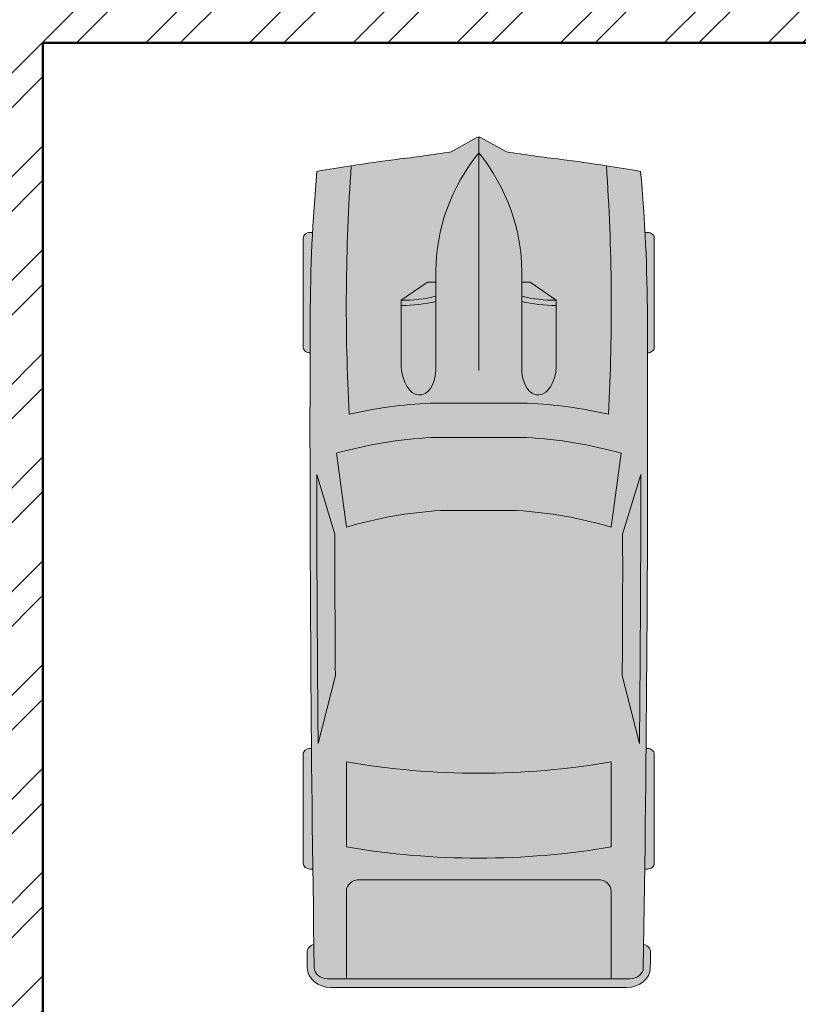
# Model space of a CAD drawing. Units: inches. Extents: x -31485 to -28799, y 18003 to 19130.
# Tile 2 of 15: x -30873 to -30771, y 18270 to 18398. Entities that reach past the tile are written whole.
import ezdxf

# ---------------------------------------------------------------- set-up
doc = ezdxf.new("R2010")
doc.units = ezdxf.units.IN
for name, color, linetype, lineweight in [('A-EQPM', 8, 'Continuous', 18), ('A-WALL', 7, 'Continuous', 50), ('A-WALL-PATT', 8, 'Continuous', 13)]:
    doc.layers.add(name, color=color, linetype=linetype, lineweight=lineweight)

# ---------------------------------------------------------------- blocks, each defined once
blk = doc.blocks.new('*U75')
for p, q in [((536.0433148737552, 950.1792138851854), (536.0433148737552, 935.5404748014407)), ((1182.463644577746, 987.7673041878503), (567.7039087844591, 987.7673041878503)), ((1214.124238488447, 949.7089586534819), (1214.124238488447, 950.1792138851854)), ((3440.463608272525, 941.6679440245914), (3440.463608272525, 950.1792138851854)), ((3472.124202183229, 987.7673041878503), (4086.88393797651, 987.767304187848)), ((4118.544531887212, 950.1792138851804), (4118.544531887212, 934.0601128753084)), ((2234.827175480885, 809.5287016048088), (1898.878785383111, 912.4126225124705)), ((3411.559256322833, 904.3494681924599), (3029.921878250559, 807.1504809911063)), ((4736.411271353851, -850.8646766016326), (4736.411271353883, 850.864676601626)), ((4785.334832293326, -832.0706314503777), (4785.334832293357, 832.0706314502926)), ((1778.76917512805, 801.0177247054045), (2194.716249451875, 745.5217224176465)), ((3515.941238262737, 745.5217224176508), (3994.062813016633, 745.5217224176508)), ((4736.411271353883, 745.5217224176529), (4242.012185201922, 745.5217224176529)), ((4178.690997380514, 670.345541812321), (4178.690997380509, -670.3455418123318)), ((819.5542361210883, 295.2827619512633), (917.6699264680983, 436.1082195367583)), ((917.6699264680983, 436.1082195367583), (1293.848362214069, 436.1082195367583)), ((815.9220749762081, 241.4481679439487), (815.9220749762081, 283.3039660446585)), ((756.2288711996046, 241.4481679439487), (1312.764151599097, 241.4481679439487)), ((1496.485716216861, -273.6820371142997), (1496.485716216861, 273.6820371142868)), ((1690.372337881975, -267.4332505757059), (1690.372337881975, 267.4332505756928)), ((4736.411271353883, -267.4332505757059), (4736.411271353883, 267.4332505756928)), ((2101.521373270556, 215.7994139342878), (2101.521373270556, -215.7994139342835)), ((82.96813941916749, 155.6585683733955), (2.596917328392246, 10.3141998552517)), ((-1.1252e-12, -6.4972e-12), (1312.764151599097, -6.4972e-12)), ((2.596917328392246, -10.31419985525964), (82.96813941916749, -155.6585683734063)), ((756.2288711996046, -241.4481679439617), (1312.764151599097, -241.4481679439617)), ((815.9220749762081, -241.4481679439617), (815.9220749762081, -283.3039660446715)), ((819.5542361210883, -295.2827619512763), (917.6699264680983, -436.1082195367712)), ((917.6699264680983, -436.1082195367712), (1293.848362214069, -436.1082195367712)), ((2194.716249451869, -745.5217224176688), (1778.769175128041, -801.0177247054262)), ((3994.062813016633, -745.5217224176616), (3515.941238262737, -745.5217224176638)), ((4242.012185201917, -745.5217224176638), (4736.411271353857, -745.5217224176594)), ((2234.827175480882, -809.5287016048153), (1898.878785383109, -912.4126225124726)), ((3411.559256322828, -904.349468192473), (3029.921878250557, -807.150480991115)), ((536.0433148737552, -950.1792138851984), (536.0433148737552, -935.5404748014537)), ((3440.463608272523, -941.6679440246044), (3440.463608272523, -950.1792138851984)), ((4118.544531887212, -950.1792138851933), (4118.544531887212, -934.0601128753214)), ((1182.463644577746, -987.7673041878633), (567.7039087844591, -987.7673041878633)), ((1214.124238488447, -949.7089586534948), (1214.124238488447, -950.1792138851984)), ((3472.124202183229, -987.7673041878633), (4086.883937976504, -987.767304187861))]:
    blk.add_line(p, q)
for centre, major_axis, ratio, start_param, end_param in [((1046.255263051279, -12467.92283887244), (3.2861e-12, 13417.14359589015), 0.8423038695439741, 0.0028100083536837, 0.0755983031096952), ((567.7039087844591, 950.1792138851861), (5.296e-13, -37.5880903026662), 0.842303869543976, 3.141592653589776, 4.712388980384677), ((1637.842620806017, -268112.68896731), (4.8454159e-09, 269062.8681811952), 0.842303869543847, -0.0133969486112073, 0.0027970409639888), ((1182.463644577746, 950.1792138851861), (5.601e-13, 37.58809030266621), 0.8423038695439758, -1.570796326794884, 1.73e-14), ((3472.124202183229, 950.1792138851861), (5.988e-12, -37.5880903026662), 0.8423038695439762, 3.141592653589603, 4.712388980384554), ((4086.88393797651, 950.179213885181), (1.4197e-12, 37.5880903026662), 0.842303869543976, -1.570796326794865, 4.44e-14), ((4587.952203166941, 910.2894362332722), (1.8792e-12, 56.38213545399769), 0.8423038695439691, -0.0130174256259048, 1.249894140392862), ((1637.84262086767, -268131.4830124673), (3.42859201765e-05, 269120.9512111412), 0.8423038681351471, -0.0133969484821159, -0.0130174254969711), ((4673.090083532448, 832.070631450172), (2.1733e-12, -133.2592106239272), 0.8423038695439737, 1.570796326795794, 3.128195704978164), ((6757.162543998887, -699.1204428451242), (4.9938223e-09, 7958.017136535005), 0.8423038695435286, 1.367075990158062, 1.391760499156098), ((1637.842620802809, -268112.6889680619), (4.87113144e-08, -269025.2800916445), 0.8423038695482963, 3.133765086725325, 3.140440689641252), ((4673.090083532475, 850.8646766015395), (7.5e-15, -75.17618060533067), 0.8423038695439952, 1.570796326796048, 3.128195704978389), ((3436.395912346701, 136.8410185571553), (5.76965e-11, 2077.023647078763), 0.8423038695439563, 1.245306111696802, 1.507880129813836), ((2433.035484508693, -93125.37499596032), (4.952654e-09, -93935.19844392464), 0.8423038695446962, 3.134048706297306, 3.14409775411291), ((951.8333444315502, -15086.63944974413), (1.5767e-12, -15832.53653317094), 0.8423038695439826, 3.09604606856106, 3.200911180495224), ((3413.769624379244, 136.8410185571329), (1.08602e-11, -2280.347340451234), 0.84230386954398, 4.44948196380473, 4.652344057257214), ((3799.722190048092, 71.1058404433382), (2.17448e-11, -2021.323467232052), 0.842303869543983, 4.372215489277867, 4.640744122441986), ((433.884764992104, -3.6096e-12), (1.7438e-12, 3734.255266801694), 0.8423038695439766, 4.511394369635731, 4.913383591133647), ((912.0063397460013, -3.6096e-12), (1.7438e-12, 3734.255266801694), 0.8423038695439766, 4.511394369635731, 4.913383591133647), ((4242.012185201922, 670.3455418123216), (3.5405e-12, 75.17618060533239), 0.842303869543976, 5.55e-14, 1.57079632679492), ((6583.045501169266, -699.1204428451198), (3.826807e-09, -7754.693443154298), 0.8423038695443791, 4.528606069860317, 4.561837674556238), ((-5194.164488957196, 1330.879982200552), (1.0466145e-09, -6374.389491984369), 0.8423038695441164, 1.385369446298923, 1.434372047871027), ((331.12799165183, 432.0470009052715), (3.125e-11, 696.3661584994836), 0.8423038695439277, 4.435146050259648, 4.718221029521873), ((360.7019022476185, 432.0470009052715), (3.125e-11, 696.3661584994836), 0.8423038695439277, 4.435146050259648, 4.718221029521873), ((1290.073045555822, 338.7781937403542), (161.0379696969085, -9.057857958340485), 0.6038335755719145, -1.39555193967809, 1.581314658479915), ((831.7523719315589, 283.3039660446593), (3.3347e-12, 18.79404515133458), 0.8423038695439091, 0.8797135699495516, 1.570796326795045), ((756.2288711996046, -1185.240851913765), (1.2998e-12, 1426.689019857713), 0.842303869543976, 7e-16, 0.5903187773915901), ((15.83029695535095, -3.6096e-12), (1.9e-15, -18.79404515133476), 0.842303869543842, 4.131459131953847, 5.293318828815531), ((756.2288711996046, 1185.240851913753), (1.01699e-11, 1426.689019857713), 0.8423038695439736, 2.55127387619821, 3.141592653589801), ((-5194.164488957196, -1330.879982200562), (1.0234792e-09, 6374.389491984348), 0.8423038695441192, -1.43437204787103, -1.385369446298926), ((3799.722190048497, -71.10584044329416), (1.038796e-10, -2021.323467232635), 0.8423038695439419, -1.499151468852248, -1.230622835688196), ((331.12799165183, -432.0470009052816), (3.1922e-11, -696.3661584994801), 0.842303869543932, 1.564964277657711, 1.848039256919935), ((360.7019022476185, -432.0470009052816), (3.1922e-11, -696.3661584994801), 0.842303869543932, 1.564964277657711, 1.848039256919935), ((3413.769624379237, -136.841018557156), (1.090899e-10, -2280.347340451348), 0.8423038695439354, -1.510751403667474, -1.307889310215002), ((3436.395912346742, -136.8410185572101), (8.13766e-11, -2077.023647078826), 0.8423038695439492, -1.50788012981387, -1.245306111696839), ((831.7523719315589, -283.3039660446737), (3.3028e-12, -18.79404515133458), 0.8423038695439093, 4.712388980384541, 5.403471737230034), ((6583.045501169163, 699.1204428449458), (2.756795e-10, 7754.693443157768), 0.8423038695439974, 1.721347632622872, 1.754579237318777), ((6757.162543998887, 699.1204428451076), (2.2231118e-09, 7958.017136528592), 0.8423038695441819, 1.749832154434603, 1.774516663432659), ((951.8333444315729, 15086.63944974408), (2.97009e-11, -15832.5365331709), 0.8423038695439528, -0.0593185269054384, 0.0455465850287298), ((4242.012185201917, -670.3455418123318), (2.579e-13, -75.17618060533128), 0.8423038695439885, 4.712388980384686, 6.283185307179581), ((2433.03548450906, 93125.37499596029), (4.1600574e-09, -93935.19844392457), 0.8423038695447548, -0.0025051005232382, 0.007543947292366), ((4673.090083532448, -850.8646766015358), (2.354e-13, 75.17618060532999), 0.8423038695439732, 3.154989602201626, 4.71238898038339), ((4673.090083532349, -832.0706314501077), (6.1679e-12, -133.2592106240062), 0.8423038695439807, 0.0133969486110846, 1.570796326792831), ((1046.255263051284, 12467.92283887242), (3.49903e-10, -13417.14359589015), 0.8423038695440652, -0.0755983031097181, -0.0028100083537155), ((1637.842620801787, 268112.6889680619), (1.55395844e-08, 269062.868181947), 0.8423038695458147, 3.138795612625926, 3.154989602201039), ((1637.842620803916, 268112.6889680615), (4.0766478e-08, -269025.280091644), 0.8423038695397146, 0.0011519639481523, 0.0078275668641468), ((4587.952203166856, -910.2894362333229), (5.777e-12, -56.38213545402103), 0.8423038695439803, -1.249894138785958, 0.0130174256254374), ((567.7039087844591, -950.1792138851977), (5.601e-13, 37.58809030266621), 0.8423038695439758, 1.570796326794908, 3.14159265358981), ((1182.463644577746, -950.1792138851977), (5.296e-13, -37.5880903026662), 0.842303869543976, -1.69e-14, 1.570796326794884), ((3472.124202183229, -950.1792138851955), (3.96e-13, -37.58809030266733), 0.8423038695440105, -1.570796326794875, -1.27e-14), ((4086.883937976504, -950.1792138851933), (5.0003e-12, 37.58809030266732), 0.8423038695440109, 3.141592653589951, 4.712388980384771), ((1637.842620726191, 268131.4830135791), (2.37878358395e-05, 269120.9512123862), 0.8423038705260315, 3.154610079306566, 3.154989602290631)]:
    blk.add_ellipse(centre, major_axis=major_axis, ratio=ratio, start_param=start_param, end_param=end_param)
at = {"extrusion": (0, 0, -1)}
blk.add_ellipse((1290.073045555822, -338.7781937403665), major_axis=(161.0379696969085, 9.057857958340424), ratio=0.6038335755719145, start_param=-1.39555193967809, end_param=1.581314658479915, dxfattribs=at)

msp = doc.modelspace()

# ---------------------------------------------------------------- hatches: boundary and pattern name
at = {"layer": 'A-EQPM'}
h = msp.add_hatch(color=256, dxfattribs=at)
h.dxf.hatch_style = 1
edge = h.paths.add_edge_path()
edge.add_ellipse((-30809.74980735968, 18303.27344922968), major_axis=(-47.91849192778267, 1.361529e-10), ratio=0.8423038695419347, start_angle=248.1650462034528, end_angle=265.722579037107)
edge.add_line((-30806.7369467095, 18343.55552145171), (-30819.07671768603, 18343.55552145171))
edge.add_ellipse((-30816.06385703584, 18303.27344922968), major_axis=(47.91849192778146, 1.460375e-10), ratio=0.8423038695419556, start_angle=94.277420962876, end_angle=111.8349537965306)
edge.add_line((-30831.3869113385, 18341.51614017747), (-30830.10657698055, 18331.91992948851))
edge.add_ellipse((-30814.54729721899, 18294.89123974947), major_axis=(46.63344704056234, 1.445442e-10), ratio=0.842303869541784, start_angle=94.8700695969602, end_angle=112.7919148774121, ccw=False)
edge.add_line((-30817.8854863836, 18334.07000511634), (-30807.92817801193, 18334.07000511634))
edge.add_ellipse((-30811.26636717653, 18294.89123974948), major_axis=(-46.63344704055716, 1.546607e-10), ratio=0.8423038695417213, start_angle=247.20808512260112, end_angle=265.1299304030565, ccw=False)
edge.add_line((-30795.70708741497, 18331.91992948851), (-30794.42675305702, 18341.51614017747))
edge = h.paths.add_edge_path()
edge.add_ellipse((-30840.2512267956, 18365.10691121584), major_axis=(-32.91478475822442, 2.78257e-11), ratio=0.8423038695443898, start_angle=180.0000000000484, end_angle=209.4385695980319)
edge.add_ellipse((-30785.56243759992, 18365.10691121584), major_axis=(32.91478475822442, 2.78184e-11), ratio=0.8423038695443903, start_angle=150.561430401968, end_angle=179.9999999999515)
edge.add_line((-30818.47722235815, 18365.10691121584), (-30818.47722235815, 18352.26722526484))
edge.add_ellipse((-30820.72269898621, 18352.79072608453), major_axis=(-0.2089715704820894, 3.715266632531377), ratio=0.6038335755718302, start_angle=89.0020142750023, end_angle=253.6574080457279, ccw=False)
edge.add_line((-30822.96817561427, 18352.70362670025), (-30822.96817561427, 18361.38234509712))
edge.add_line((-30822.96817561427, 18361.38234509712), (-30819.64068913299, 18363.70066622193))
edge.add_ellipse((-30819.44286698441, 18363.36452746144), major_axis=(0.4335927047225755, 4.12191e-11), ratio=0.8423038695061222, start_angle=89.99999999455332, end_angle=134.4802108771379, ccw=False)
edge.add_line((-30819.44286698441, 18363.72974427442), (-30818.47722235815, 18363.72974427442))
edge.add_line((-30818.47722235815, 18363.72974427442), (-30818.47722235815, 18365.10691121584))
edge.add_ellipse((-30785.56243759992, 18365.10691121584), major_axis=(32.91478475822442, 2.78184e-11), ratio=0.8423038695443903, start_angle=150.5614304019681, end_angle=179.9999999999516, ccw=False)
edge.add_line((-30812.90683219776, 18380.53894657792), (-30812.90683219776, 18382.55367794428))
edge.add_ellipse((-30812.90683219776, 18382.18846113131), major_axis=(-0.4335927046986816, 0), ratio=0.842303869552539, start_angle=270, end_angle=307.9331304600232)
edge.add_line((-30813.14478851723, 18382.49376511555), (-30816.49799201077, 18380.63954079683))
edge.add_ellipse((-30843.61123066403, 18502.38694488138), major_axis=(-147.0619421372835, 4.9907306e-09), ratio=0.8423038695736066, start_angle=99.2565660091451, end_angle=102.55493264608151, ccw=False)
edge.add_ellipse((-30796.77759970489, 18230.67788531626), major_axis=(178.9065886092977, 1.2789651e-09), ratio=0.8423038695391513, start_angle=100.209538996733, end_angle=102.4446272930335)
edge.add_ellipse((-30464.84675512309, 18360.59416944481), major_axis=(365.2684817172171, 7.18011e-11), ratio=0.8423038695434502, start_angle=177.1362853921513, end_angle=182.1985405659441)
edge.add_ellipse((-30816.06385703584, 18303.79545464779), major_axis=(52.60932189168197, 7.16232e-11), ratio=0.8423038695431074, start_angle=94.08241069107589, end_angle=107.71995322267611, ccw=False)
edge.add_line((-30819.22088187392, 18348.02863109984), (-30806.59278252161, 18348.02863109984))
edge.add_ellipse((-30809.74980735968, 18303.79545464779), major_axis=(-52.6093218916263, 2.96862e-11), ratio=0.842303869543985, start_angle=252.2800467772827, end_angle=265.9175893088832, ccw=False)
edge.add_ellipse((-31160.96690927244, 18360.59416944481), major_axis=(365.2684817172168, 5.54988e-11), ratio=0.8423038695419378, start_angle=-2.198540565964143, end_angle=2.863714607828726)
edge.add_ellipse((-30829.03606469064, 18230.67788531626), major_axis=(-178.9065886093012, 1.2581094e-09), ratio=0.8423038695391548, start_angle=257.5553727069574, end_angle=259.7904610032577)
edge.add_ellipse((-30782.2024337315, 18502.38694488138), major_axis=(147.0619421407358, 1.9919546e-09), ratio=0.8423038695542743, start_angle=257.4450673550873, end_angle=260.74343399202326, ccw=False)
edge.add_line((-30809.31567238475, 18380.63954079683), (-30812.6688758783, 18382.49376511555))
edge.add_ellipse((-30812.90683219776, 18382.18846113131), major_axis=(-0.4335927046986816, 0), ratio=0.842303869552539, start_angle=232.0668695399768, end_angle=270)
edge.add_line((-30812.90683219776, 18382.55367794428), (-30812.90683219776, 18380.53894657792))
edge.add_ellipse((-30840.2512267956, 18365.10691121584), major_axis=(-32.91478475822442, 2.78257e-11), ratio=0.8423038695443898, start_angle=180.0000000000485, end_angle=209.438569598032, ccw=False)
edge.add_line((-30807.33644203738, 18365.10691121584), (-30807.33644203738, 18363.72974427442))
edge.add_line((-30807.33644203738, 18363.72974427442), (-30806.21471099341, 18363.72974427442))
edge.add_line((-30806.21471099341, 18363.72974427442), (-30802.84548878126, 18361.38234509712))
edge.add_line((-30802.84548878126, 18361.38234509712), (-30802.84548878126, 18352.70362670025))
edge.add_ellipse((-30805.09096540932, 18352.79072608453), major_axis=(0.2089715704820894, 3.715266632531377), ratio=0.6038335755718302, start_angle=106.3425919542722, end_angle=270.9979857249977, ccw=False)
edge.add_line((-30807.33644203738, 18352.26722526484), (-30807.33644203738, 18365.10691121584))
edge = h.paths.add_edge_path()
edge.add_ellipse((-28664.43464880163, 18326.42172615445), major_axis=(-2167.155417170912, 9.004676e-10), ratio=0.8423038695746358, start_angle=-0.12089736900918524, end_angle=0.3640763489138976, ccw=False)
edge.add_line((-30831.58326595316, 18330.99454036844), (-30833.95687510317, 18338.74512146637))
edge.add_ellipse((-24627.34619108991, 18344.76742138713), major_axis=(6206.614802166701, 5.2511138e-09), ratio=0.842303869515611, start_angle=180.0555943134505, end_angle=180.377764193861)
edge.add_line((-30833.77085209099, 18303.84644949518), (-30831.52839862151, 18312.65110978209))
edge = h.paths.add_edge_path()
edge.add_ellipse((-36998.46747330562, 18344.76742138716), major_axis=(-6206.61480216671, 6.192387e-09), ratio=0.8423038695127218, start_angle=179.6222358061472, end_angle=179.9444056865578)
edge.add_line((-30791.85678929235, 18338.74512146637), (-30794.23039844237, 18330.99454036844))
edge.add_ellipse((-32961.37901559391, 18326.42172615446), major_axis=(-2167.155417170919, 1.3253717e-09), ratio=0.8423038695188795, start_angle=179.6359236511448, end_angle=180.1208973690678, ccw=False)
edge.add_line((-30794.28526577401, 18312.65110978209), (-30792.04281230453, 18303.84644949516))
edge = h.paths.add_edge_path()
edge.add_ellipse((-30812.90683219776, 18372.54363129024), major_axis=(-86.15206721880882, 2.44e-14), ratio=0.8423038695434939, start_angle=76.40186530976911, end_angle=103.598134690231, ccw=False)
edge.add_line((-30830.10657698055, 18301.43827895458), (-30830.10657698055, 18290.40765595108))
edge.add_ellipse((-30812.90683219776, 18361.51300828673), major_axis=(-86.15206721880666, 5.3e-15), ratio=0.8423038695434728, start_angle=76.40186530976838, end_angle=103.5981346902316)
edge.add_line((-30795.70708741497, 18290.40765595108), (-30795.70708741497, 18301.43827895458))
edge = h.paths.add_edge_path()
edge.add_ellipse((-30797.44145823379, 18284.68727813726), major_axis=(-1.734370818820025, 1.15572e-11), ratio=0.8423038695444475, start_angle=180.0000000003817, end_angle=270.0000000003818)
edge.add_line((-30797.44145823379, 18286.14814538917), (-30828.37220616173, 18286.14814538917))
edge.add_ellipse((-30828.37220616173, 18284.68727813726), major_axis=(1.734370818820025, 1.15576e-11), ratio=0.8423038695444475, start_angle=89.99999999961817, end_angle=179.9999999996181)
edge.add_line((-30830.10657698055, 18284.68727813726), (-30830.10657698055, 18273.28112074847))
edge.add_line((-30830.10657698055, 18273.28112074847), (-30795.70708741497, 18273.28112074847))
edge.add_line((-30795.70708741497, 18273.28112074847), (-30795.70708741497, 18284.68727813726))
h = msp.add_hatch(color=256, dxfattribs=at)
h.dxf.hatch_style = 1
edge = h.paths.add_edge_path()
edge.add_ellipse((-36998.46747328827, 18344.76742138709), major_axis=(6207.481987558777, 4.152598e-10), ratio=0.8423038695472291, start_angle=-0.3838667787963557, end_angle=0.0902290885904627)
edge.add_ellipse((-36998.46747328827, 18344.76742138709), major_axis=(6207.481987558777, 4.152598e-10), ratio=0.8423038695472291, start_angle=0.0902290885904627, end_angle=0.1349865768543979)
edge.add_ellipse((-31100.55115475978, 18358.41578502847), major_axis=(309.5435567121417, 3.12922e-11), ratio=0.8423038695440732, start_angle=0.1806905311799308, end_angle=2.179950313639523)
edge.add_ellipse((-31100.55115475978, 18358.41578502847), major_axis=(309.5435567121417, 3.12922e-11), ratio=0.8423038695440732, start_angle=2.179950313639523, end_angle=3.650427585692763)
edge.add_ellipse((-30829.03606469064, 18226.66087466593), major_axis=(183.5974185536168, 2.07254122e-08), ratio=0.8423038696260594, start_angle=76.2194710040335, end_angle=77.87403444124779)
edge.add_ellipse((-31160.96690927244, 18360.59416944481), major_axis=(365.2684817172168, 5.54988e-11), ratio=0.8423038695419378, start_angle=-2.1985405659640946, end_angle=2.8637146078286833, ccw=False)
edge.add_ellipse((-30809.74980735968, 18303.79545464779), major_axis=(-52.6093218916263, 2.96862e-11), ratio=0.842303869543985, start_angle=252.2800467772827, end_angle=265.9175893088831)
edge.add_line((-30806.59278252161, 18348.02863109984), (-30819.22088187392, 18348.02863109984))
edge.add_ellipse((-30816.06385703584, 18303.79545464779), major_axis=(52.60932189168197, 7.16232e-11), ratio=0.8423038695431074, start_angle=94.08241069107586, end_angle=107.719953222676)
edge.add_ellipse((-30464.84675512309, 18360.59416944481), major_axis=(365.2684817172171, 7.18011e-11), ratio=0.8423038695434502, start_angle=177.1362853921513, end_angle=182.1985405659441, ccw=False)
edge.add_ellipse((-30796.77759970488, 18226.66087466593), major_axis=(-183.5974185535601, 2.07797544e-08), ratio=0.8423038696263095, start_angle=-77.87403444123211, end_angle=-76.21947100401783)
edge.add_ellipse((-30525.26250963575, 18358.41578502847), major_axis=(-309.5435567121417, 3.20483e-11), ratio=0.8423038695440663, start_angle=-3.650427585692615, end_angle=-2.179950313639383)
edge.add_ellipse((-30525.26250963575, 18358.41578502847), major_axis=(-309.5435567121417, 3.20483e-11), ratio=0.8423038695440663, start_angle=-2.179950313639383, end_angle=-0.1356123904320413)
edge.add_ellipse((-24627.3461910899, 18344.76742138718), major_axis=(6207.481987576122, 7.89454e-11), ratio=0.842303869542251, start_angle=179.8650134231422, end_angle=179.9097709114061)
edge.add_ellipse((-24627.3461910899, 18344.76742138718), major_axis=(6207.481987576122, 7.89454e-11), ratio=0.842303869542251, start_angle=179.9097709114061, end_angle=180.3838667787915)
edge.add_ellipse((-24627.3461910899, 18344.76742138718), major_axis=(6207.481987576122, 7.89454e-11), ratio=0.842303869542251, start_angle=180.3838667787915, end_angle=180.5282714718166)
edge.add_ellipse((-24627.3461910899, 18344.76742138718), major_axis=(6207.481987576122, 7.89454e-11), ratio=0.842303869542251, start_angle=180.5282714718166, end_angle=180.6465540970602)
edge.add_ellipse((-30832.53691787089, 18274.74198800039), major_axis=(1.734370818820398, 6.2835e-12), ratio=0.8423038695442665, start_angle=180.6465540968934, end_angle=269.9999999996497)
edge.add_line((-30832.53691787089, 18273.28112074847), (-30830.10657698055, 18273.28112074847))
edge.add_line((-30830.10657698055, 18273.28112074847), (-30830.10657698055, 18285.22199266301))
edge.add_ellipse((-30828.37220616173, 18284.68727813726), major_axis=(1.734370818820025, 1.15576e-11), ratio=0.8423038695444475, start_angle=89.99999999961818, end_angle=179.9999999996182, ccw=False)
edge.add_line((-30828.37220616173, 18286.14814538917), (-30796.80663445453, 18286.14814538917))
edge.add_ellipse((-30797.44145823379, 18284.68727813726), major_axis=(-1.734370818820025, 1.15572e-11), ratio=0.8423038695444475, start_angle=180.0000000003818, end_angle=270.00000000038176, ccw=False)
edge.add_line((-30795.70708741497, 18284.68727813726), (-30795.70708741497, 18273.28112074847))
edge.add_line((-30795.70708741497, 18273.28112074847), (-30793.27674652463, 18273.28112074847))
edge.add_ellipse((-30793.27674652464, 18274.74198800038), major_axis=(-1.734370818820364, 1.2413e-12), ratio=0.8423038695421853, start_angle=90.00000000018369, end_angle=179.3534459030602)
edge.add_ellipse((-36998.46747328827, 18344.76742138709), major_axis=(6207.481987558777, 4.152598e-10), ratio=0.8423038695472291, start_angle=-0.6465540970657812, end_angle=-0.618643196323059)
edge.add_ellipse((-36998.46747328827, 18344.76742138709), major_axis=(6207.481987558777, 4.152598e-10), ratio=0.8423038695472291, start_angle=-0.618643196323059, end_angle=-0.528271471821792)
edge.add_ellipse((-36998.46747328827, 18344.76742138709), major_axis=(6207.481987558777, 4.152598e-10), ratio=0.8423038695472291, start_angle=-0.528271471821792, end_angle=-0.3838667787963557)
edge = h.paths.add_edge_path(flags=16)
edge.add_ellipse((-30814.54729721899, 18294.89123974947), major_axis=(46.63344704056234, 1.445442e-10), ratio=0.842303869541784, start_angle=94.8700695969603, end_angle=112.7919148774121)
edge.add_line((-30830.10657698055, 18331.91992948851), (-30831.3869113385, 18341.51614017747))
edge.add_ellipse((-30816.06385703584, 18303.27344922968), major_axis=(47.91849192778146, 1.460375e-10), ratio=0.8423038695419556, start_angle=94.27742096287608, end_angle=111.8349537965307, ccw=False)
edge.add_line((-30819.07671768603, 18343.55552145171), (-30806.7369467095, 18343.55552145171))
edge.add_ellipse((-30809.74980735968, 18303.27344922968), major_axis=(-47.91849192778267, 1.361529e-10), ratio=0.8423038695419347, start_angle=248.1650462034528, end_angle=265.72257903710704, ccw=False)
edge.add_line((-30794.42675305702, 18341.51614017747), (-30795.70708741497, 18331.91992948851))
edge.add_ellipse((-30811.26636717653, 18294.89123974948), major_axis=(-46.63344704055716, 1.546607e-10), ratio=0.8423038695417213, start_angle=247.208085122601, end_angle=265.1299304030565)
edge.add_line((-30807.92817801193, 18334.07000511634), (-30817.8854863836, 18334.07000511634))
edge = h.paths.add_edge_path(flags=16)
edge.add_line((-30794.23039844237, 18330.99454036844), (-30791.85678929235, 18338.74512146637))
edge.add_ellipse((-36998.46747330562, 18344.76742138716), major_axis=(-6206.61480216671, 6.192387e-09), ratio=0.8423038695127218, start_angle=179.6222358061473, end_angle=179.9444056865578, ccw=False)
edge.add_line((-30792.04281230453, 18303.84644949516), (-30794.28526577401, 18312.65110978209))
edge.add_ellipse((-32961.37901559391, 18326.42172615446), major_axis=(-2167.155417170919, 1.3253717e-09), ratio=0.8423038695188795, start_angle=179.6359236511447, end_angle=180.1208973690677)
edge = h.paths.add_edge_path(flags=16)
edge.add_ellipse((-28664.43464880163, 18326.42172615445), major_axis=(-2167.155417170912, 9.004676e-10), ratio=0.8423038695746358, start_angle=-0.1208973690091865, end_angle=0.364076348913875)
edge.add_line((-30831.52839862151, 18312.65110978209), (-30833.77085209099, 18303.84644949518))
edge.add_ellipse((-24627.34619108991, 18344.76742138713), major_axis=(6206.614802166701, 5.2511138e-09), ratio=0.842303869515611, start_angle=180.0555943134506, end_angle=180.3777641938611, ccw=False)
edge.add_line((-30833.95687510317, 18338.74512146637), (-30831.58326595316, 18330.99454036844))
edge = h.paths.add_edge_path(flags=16)
edge.add_ellipse((-30812.90683219776, 18372.54363129024), major_axis=(-86.15206721880882, 2.44e-14), ratio=0.8423038695434939, start_angle=76.40186530976904, end_angle=103.5981346902309)
edge.add_line((-30795.70708741497, 18301.43827895458), (-30795.70708741497, 18290.40765595108))
edge.add_ellipse((-30812.90683219776, 18361.51300828673), major_axis=(-86.15206721880666, 5.3e-15), ratio=0.8423038695434728, start_angle=76.40186530976843, end_angle=103.59813469023157, ccw=False)
edge.add_line((-30830.10657698055, 18290.40765595108), (-30830.10657698055, 18301.43827895458))
h = msp.add_hatch(color=256, dxfattribs=at)
h.dxf.hatch_style = 1
edge = h.paths.add_edge_path()
edge.add_ellipse((-30802.9391841383, 18374.9143070506), major_axis=(-16.06568908915088, 3.60949e-11), ratio=0.8423038695435023, start_angle=71.33250450753093, end_angle=90.39670986011208, ccw=False)
edge.add_line((-30807.33644203738, 18361.89885908758), (-30807.33644203738, 18361.21656680932))
edge.add_ellipse((-30802.9391841383, 18374.23201477234), major_axis=(16.06568908904641, 9.1463e-11), ratio=0.8423038695487669, start_angle=251.332504507076, end_angle=270.3967098596572)
edge.add_line((-30802.84548878126, 18360.70005281887), (-30802.84548878126, 18361.38234509712))
edge = h.paths.add_edge_path()
edge.add_ellipse((-30822.87448025722, 18374.9143070506), major_axis=(16.06568908915091, 3.60949e-11), ratio=0.8423038695435009, start_angle=269.6032901398879, end_angle=288.667495492469, ccw=False)
edge.add_line((-30822.96817561427, 18361.38234509712), (-30822.96817561427, 18360.70005281887))
edge.add_ellipse((-30822.87448025722, 18374.23201477234), major_axis=(-16.06568908904639, 9.1463e-11), ratio=0.8423038695487673, start_angle=89.60329014034272, end_angle=108.667495492924)
edge.add_line((-30818.47722235815, 18361.21656680932), (-30818.47722235815, 18361.89885908758))
edge = h.paths.add_edge_path()
edge.add_ellipse((-30790.9854857295, 18369.45632336739), major_axis=(0.8671854094100124, 1.6795e-12), ratio=0.8423038695444477, start_angle=-1.109639e-10, end_angle=89.99999999988906)
edge.add_line((-30790.9854857295, 18370.18675699335), (-30791.3232124095, 18370.18675699335))
edge.add_ellipse((-31100.55115475978, 18358.41578502847), major_axis=(309.5435567121417, 3.12922e-11), ratio=0.8423038695440732, start_angle=0.18069053117989142, end_angle=2.1799503136394947, ccw=False)
edge.add_ellipse((-31100.55115475978, 18358.41578502847), major_axis=(309.5435567121417, 3.12922e-11), ratio=0.8423038695440732, start_angle=0.1356123904321862, end_angle=0.18069053117989142, ccw=False)
edge.add_ellipse((-36998.46747328827, 18344.76742138709), major_axis=(6207.481987558777, 4.152598e-10), ratio=0.8423038695472291, start_angle=0.09022908859049039, end_angle=0.13498657685437365, ccw=False)
edge.add_line((-30790.99633487007, 18354.54292197479), (-30790.9854857295, 18354.54292197479))
edge.add_ellipse((-30790.9854857295, 18355.27335560075), major_axis=(-0.8671854094100128, 1.6795e-12), ratio=0.8423038695444475, start_angle=90.00000000011094, end_angle=180.0000000001109)
edge.add_line((-30790.11830032009, 18355.27335560075), (-30790.11830032009, 18369.45632336739))
edge = h.paths.add_edge_path()
edge.add_ellipse((-30525.26250963575, 18358.41578502847), major_axis=(-309.5435567121417, 3.20483e-11), ratio=0.8423038695440663, start_angle=-2.179950313639381, end_angle=-0.13561239043201567, ccw=False)
edge.add_line((-30834.49045198602, 18370.18675699335), (-30834.82817866603, 18370.18675699335))
edge.add_ellipse((-30834.82817866603, 18369.45632336739), major_axis=(-0.8671854094100128, 1.6795e-12), ratio=0.8423038695444475, start_angle=-89.99999999988903, end_angle=1.109639e-10)
edge.add_line((-30835.69536407544, 18369.45632336739), (-30835.69536407544, 18355.27335560075))
edge.add_ellipse((-30834.82817866603, 18355.27335560075), major_axis=(0.8671854094100124, 1.6795e-12), ratio=0.8423038695444477, start_angle=179.999999999889, end_angle=269.999999999889)
edge.add_line((-30834.82817866603, 18354.54292197479), (-30834.81732952545, 18354.54292197479))
edge.add_ellipse((-24627.3461910899, 18344.76742138718), major_axis=(6207.481987576122, 7.89454e-11), ratio=0.842303869542251, start_angle=179.8650134231423, end_angle=179.9097709114062, ccw=False)
edge = h.paths.add_edge_path()
edge.add_ellipse((-30793.71033922934, 18274.74198800039), major_axis=(3.074389845080431, 4.5193e-12), ratio=0.8423038695441155, start_angle=269.9999999999962, end_angle=359.3534459027799)
edge.add_ellipse((-36998.90106599311, 18344.76742138567), major_axis=(6208.822006597157, 5.2733581016e-06), ratio=0.8423038788855699, start_angle=-0.6465541457119849, end_angle=-0.6282372648788389)
edge.add_ellipse((-30791.90577279079, 18276.70618269733), major_axis=(-1.30077811411332, 2.65586e-11), ratio=0.8423038695457158, start_angle=179.3717627849924, end_angle=248.4647566023133)
edge.add_ellipse((-36998.46747328827, 18344.76742138709), major_axis=(6207.481987558777, 4.152598e-10), ratio=0.8423038695472291, start_angle=-0.6465540970658026, end_angle=-0.6186431963230916, ccw=False)
edge.add_ellipse((-30793.27674652464, 18274.74198800038), major_axis=(-1.734370818820364, 1.2413e-12), ratio=0.8423038695421853, start_angle=90.00000000018372, end_angle=179.3534459030602, ccw=False)
edge.add_line((-30793.27674652463, 18273.28112074847), (-30832.53691787089, 18273.28112074847))
edge.add_ellipse((-30832.53691787089, 18274.74198800039), major_axis=(1.734370818820398, 6.2835e-12), ratio=0.8423038695442665, start_angle=180.6465540968934, end_angle=269.99999999964973, ccw=False)
edge.add_ellipse((-24627.3461910899, 18344.76742138718), major_axis=(6207.481987576122, 7.89454e-11), ratio=0.842303869542251, start_angle=180.5282714718167, end_angle=180.6465540970602, ccw=False)
edge.add_ellipse((-30833.90789160473, 18276.70618269733), major_axis=(1.300778114113422, 3.7711e-12), ratio=0.8423038695465029, start_angle=111.5352435038071, end_angle=180.6282372160113)
edge.add_ellipse((-24626.91259837676, 18344.76742138893), major_axis=(-6208.822006624284, 5.909233014e-06), ratio=0.842303880027109, start_angle=0.6282372707742053, end_angle=0.6465541516072572)
edge.add_ellipse((-30832.10332516618, 18274.74198800039), major_axis=(-3.074389845084005, 2.9376e-12), ratio=0.8423038695431365, start_angle=0.6465540971220629, end_angle=89.99999999989375)
edge.add_line((-30832.10332516619, 18272.15241753739), (-30793.71033922934, 18272.15241753739))
edge = h.paths.add_edge_path()
edge.add_ellipse((-24627.3461910899, 18344.76742138718), major_axis=(6207.481987576122, 7.89454e-11), ratio=0.842303869542251, start_angle=180.3838667787916, end_angle=180.5282714718167, ccw=False)
edge.add_line((-30834.63181729253, 18303.1796044366), (-30834.82817866603, 18303.1796044366))
edge.add_ellipse((-30834.82817866603, 18302.44917081064), major_axis=(-0.8671854094100128, 1.6795e-12), ratio=0.8423038695444475, start_angle=-89.99999999988903, end_angle=1.109639e-10)
edge.add_line((-30835.69536407544, 18302.44917081064), (-30835.69536407544, 18288.266203044))
edge.add_ellipse((-30834.82817866603, 18288.266203044), major_axis=(-0.8671854094100128, 3.5068e-12), ratio=0.8423038695402523, start_angle=2.317008e-10, end_angle=90.0000000002317)
edge.add_line((-30834.82817866603, 18287.53576941804), (-30834.4562989271, 18287.53576941804))
edge = h.paths.add_edge_path()
edge.add_ellipse((-30790.9854857295, 18302.44917081064), major_axis=(0.8671854094100124, 1.6795e-12), ratio=0.8423038695444477, start_angle=-1.109639e-10, end_angle=89.99999999988906)
edge.add_line((-30790.9854857295, 18303.1796044366), (-30791.18184710298, 18303.1796044366))
edge.add_ellipse((-36998.46747328827, 18344.76742138709), major_axis=(6207.481987558777, 4.152598e-10), ratio=0.8423038695472291, start_angle=-0.5282714718218244, end_angle=-0.38386677879640274, ccw=False)
edge.add_line((-30791.35736546843, 18287.53576941804), (-30790.9854857295, 18287.53576941804))
edge.add_ellipse((-30790.9854857295, 18288.266203044), major_axis=(0.8671854094100124, 3.5068e-12), ratio=0.8423038695402528, start_angle=269.9999999997683, end_angle=359.9999999997682)
edge.add_line((-30790.11830032009, 18288.266203044), (-30790.11830032009, 18302.44917081064))
h = msp.add_hatch(color=256, dxfattribs=at)
h.dxf.hatch_style = 1
edge = h.paths.add_edge_path()
edge.add_ellipse((-30802.9391841383, 18374.23201477234), major_axis=(16.06568908904641, 9.1463e-11), ratio=0.8423038695487669, start_angle=251.332504507076, end_angle=270.3967098596572, ccw=False)
edge.add_line((-30807.33644203738, 18361.21656680932), (-30807.33644203738, 18352.26722526484))
edge.add_ellipse((-30805.09096540932, 18352.79072608453), major_axis=(0.2089715704820894, 3.715266632531377), ratio=0.6038335755718302, start_angle=106.3425919542721, end_angle=270.9979857249977)
edge.add_line((-30802.84548878126, 18352.70362670025), (-30802.84548878126, 18360.70005281887))
edge = h.paths.add_edge_path()
edge.add_line((-30818.47722235815, 18363.72974427442), (-30819.44286698441, 18363.72974427442))
edge.add_ellipse((-30819.44286698441, 18363.36452746144), major_axis=(0.4335927047225755, 4.12191e-11), ratio=0.8423038695061222, start_angle=89.99999999455322, end_angle=134.4802108771379)
edge.add_line((-30819.71922678212, 18363.6459475951), (-30822.96817561427, 18361.38234509712))
edge.add_ellipse((-30822.87448025722, 18374.9143070506), major_axis=(16.06568908915091, 3.60949e-11), ratio=0.8423038695435009, start_angle=269.6032901398879, end_angle=288.6674954924691)
edge.add_line((-30818.47722235815, 18361.89885908758), (-30818.47722235815, 18363.72974427442))
edge = h.paths.add_edge_path()
edge.add_ellipse((-30822.87448025722, 18374.23201477234), major_axis=(-16.06568908904639, 9.1463e-11), ratio=0.8423038695487673, start_angle=89.60329014034278, end_angle=108.66749549292399, ccw=False)
edge.add_line((-30822.96817561427, 18360.70005281887), (-30822.96817561427, 18352.70362670025))
edge.add_ellipse((-30820.72269898621, 18352.79072608453), major_axis=(-0.2089715704820894, 3.715266632531377), ratio=0.6038335755718302, start_angle=89.00201427500228, end_angle=253.6574080457278)
edge.add_line((-30818.47722235815, 18352.26722526484), (-30818.47722235815, 18361.21656680932))
edge = h.paths.add_edge_path()
edge.add_ellipse((-30806.37079741112, 18363.36452746144), major_axis=(-0.4335927047225754, 4.1219e-11), ratio=0.8423038695061223, start_angle=225.5197891228621, end_angle=270.0000000054467)
edge.add_line((-30806.37079741112, 18363.72974427442), (-30807.33644203738, 18363.72974427442))
edge.add_line((-30807.33644203738, 18363.72974427442), (-30807.33644203738, 18361.89885908758))
edge.add_ellipse((-30802.9391841383, 18374.9143070506), major_axis=(-16.06568908915088, 3.60949e-11), ratio=0.8423038695435023, start_angle=71.33250450753091, end_angle=90.39670986011207)
edge.add_line((-30802.84548878126, 18361.38234509712), (-30806.0944376134, 18363.6459475951))
at = {"layer": 'A-WALL-PATT'}
h = msp.add_hatch(dxfattribs=at)
h.set_pattern_fill('ANSI32', color=256)
h.set_pattern_definition([(45, (-1687.357050595019, -0.3129728357926069), (-6.735192090801865, 6.735192090801866), []), (45, (-1682.866920595021, -0.3129728357926069), (-6.735192090801865, 6.735192090801866), [])])
h.paths.add_polyline_path([(-31156.52828769349, 18823.80296009311), (-31209.52828769349, 18823.80296009311), (-31209.52828769349, 18761.80296009311), (-31200.52828769349, 18761.80296009311), (-31200.52828769349, 18814.80296009311), (-31156.52828769349, 18814.80296009311)], flags=17)
h.paths.add_polyline_path([(-31022.5282876935, 18823.80296009311), (-31118.52828769349, 18823.80296009311), (-31118.52828769349, 18814.80296009311), (-31074.52828769349, 18814.80296009311), (-31074.52828769349, 18720.78574754094), (-31070.95696393926, 18720.78574754094), (-31068.52828769349, 18720.75952290947), (-31068.52828769349, 18814.80296009311), (-31022.5282876935, 18814.80296009311)], flags=17)
h.paths.add_polyline_path([(-30754.52828769349, 18823.80296009311), (-30850.5282876935, 18823.80296009311), (-30850.5282876935, 18814.80296009311), (-30806.5282876935, 18814.80296009311), (-30806.52828769349, 18723.10029278397), (-30800.5282876935, 18723.10029278397), (-30800.5282876935, 18814.80296009311), (-30754.52828769349, 18814.80296009311)], flags=17)
h.paths.add_polyline_path([(-30661.52828769349, 18823.80296009311), (-30716.52828769349, 18823.80296009311), (-30716.52828769349, 18814.80296009311), (-30670.52828769349, 18814.80296009311), (-30670.52828769349, 18761.80296009311), (-30661.52828769349, 18761.80296009311)], flags=17)
h.paths.add_polyline_path([(-30986.91891278487, 18670.80296009311), (-31068.52828769349, 18670.80296009311), (-31068.52828769349, 18684.75952290947), (-31074.52828769349, 18684.75952290947), (-31074.52828769349, 18670.80296009311), (-31200.52828769349, 18670.80296009311), (-31200.52828769349, 18723.80296009311), (-31209.52828769349, 18723.80296009311), (-31209.52828769349, 18641.80296009311), (-31200.52828769349, 18641.80296009311), (-31200.52828769349, 18664.80296009311), (-31104.52828769349, 18664.80296009311), (-31104.52828769349, 18628.92834044014), (-31098.52828769349, 18628.92834044014), (-31098.52828769348, 18664.8029600931), (-30986.91891278488, 18664.8029600931)], flags=17)
h.paths.add_polyline_path([(-30661.52828769349, 18723.80296009311), (-30670.52828769349, 18723.80296009311), (-30670.52828769349, 18670.80296009311), (-30800.5282876935, 18670.80296009311), (-30800.5282876935, 18687.10029278396), (-30806.52828769349, 18687.10029278396), (-30806.52828769349, 18670.80296009311), (-30885.59628027248, 18670.80296009311), (-30885.59628027248, 18667.80293426455), (-30885.59628027248, 18664.80296009311), (-30760.52828769349, 18664.80296009311), (-30760.52828769349, 18625.80296009311), (-30754.52828769349, 18625.80296009311), (-30754.52828769349, 18664.80296009311), (-30670.52828769349, 18664.80296009311), (-30670.52828769349, 18641.80296009311), (-30661.52828769349, 18641.80296009311)], flags=17)
h.paths.add_polyline_path([(-31200.52828769349, 18574.80296009311), (-31188.56436894977, 18574.80296009311), (-31188.56436894977, 18580.80296009311), (-31200.52828769349, 18580.80296009311), (-31200.52828769349, 18603.80296009311), (-31209.52828769349, 18603.80296009311), (-31209.52828769349, 18557.80296009311), (-31200.52828769349, 18557.80296009311)], flags=17)
h.paths.add_polyline_path([(-31098.52828769349, 18592.92834044014), (-31104.52828769349, 18592.92834044014), (-31104.52828769349, 18580.80296009311), (-31164.56436894977, 18580.80296009311), (-31164.56436894977, 18574.80296009311), (-31104.52828769349, 18574.80296009311), (-31104.52828769349, 18514.80296009311), (-31200.52828769349, 18514.80296009311), (-31200.52828769349, 18531.80296009311), (-31209.52828769349, 18531.80296009311), (-31209.52828769349, 18473.80296009311), (-31200.52828769349, 18473.80296009311), (-31200.52828769349, 18508.80296009311), (-31056.52828769349, 18508.80296009312), (-31056.52828769349, 18501.62307445529), (-31050.52828769349, 18501.62307445529), (-31050.52828769349, 18514.80296009311), (-31098.52828769349, 18514.80296009311)], flags=17)
h.paths.add_polyline_path([(-30661.52828769349, 18531.80296009311), (-30670.52828769349, 18531.80296009311), (-30670.52828769349, 18514.80296009311), (-30754.52828769349, 18514.80296009311), (-30754.52828769349, 18574.80296009311), (-30700.74522746605, 18574.80296009311), (-30700.74522746605, 18577.44024221289), (-30700.74522746605, 18580.8029600931), (-30754.52828769349, 18580.80296009311), (-30754.52828769349, 18589.80296009311), (-30760.52828769349, 18589.80296009311), (-30760.52828769349, 18514.80296009311), (-30820.52828769349, 18514.80296009311), (-30820.52828769348, 18499.26438911774), (-30814.52828769349, 18499.26438911774), (-30814.52828769349, 18508.80296009311), (-30670.52828769349, 18508.80296009311), (-30670.52828769349, 18473.80296009311), (-30661.52828769349, 18473.80296009311)], flags=17)
h.paths.add_polyline_path([(-30661.52828769349, 18435.80296009311), (-30670.52828769349, 18435.80296009311), (-30670.52828769349, 18400.80296009311), (-30814.52828769349, 18400.80296009311), (-30814.52828769349, 18413.15176302367), (-30820.52828769349, 18413.15176302367), (-30820.52828769349, 18400.80296009311), (-30932.52828769349, 18400.80296009311), (-30932.52828769349, 18664.80296009311), (-30921.59628027248, 18664.80296009311), (-30921.59628027248, 18670.80296009311), (-30932.5282876935, 18670.80296009311), (-30932.5282876935, 18814.80296009311), (-30888.5282876935, 18814.80296009311), (-30888.5282876935, 18823.80296009311), (-30984.5282876935, 18823.80296009311), (-30984.5282876935, 18814.80296009311), (-30938.5282876935, 18814.80296009311), (-30938.5282876935, 18670.80296009311), (-30950.91891278487, 18670.80296009311), (-30950.91891278488, 18664.80296009311), (-30938.5282876935, 18664.80296009311), (-30938.52828769349, 18400.80296009311), (-31050.52828769349, 18400.80296009311), (-31050.52828769349, 18411.18080736427), (-31056.52828769348, 18411.18080736427), (-31056.52828769348, 18400.80296009311), (-31200.52828769349, 18400.80296009311), (-31200.52828769349, 18435.80296009311), (-31209.52828769349, 18435.80296009311), (-31209.52828769349, 18179.80296009311), (-31200.52828769349, 18179.80296009311), (-31200.52828769349, 18394.80296009311), (-31001.52828769348, 18394.80296009311), (-31001.52828769348, 18179.80296009311), (-30954.52828769347, 18179.80296009311), (-30954.52828769347, 18188.80296009311), (-30995.52828769348, 18188.80296009311), (-30995.52828769348, 18394.80296009311), (-30875.52828769348, 18394.80296009311), (-30875.52828769348, 18188.80296009311), (-30916.52828769347, 18188.80296009311), (-30916.52828769347, 18179.80296009311), (-30869.52828769348, 18179.80296009311), (-30869.52828769348, 18394.80296009311), (-30670.52828769349, 18394.80296009311), (-30670.52828769349, 18179.80296009311), (-30661.52828769349, 18179.80296009311)])

# ---------------------------------------------------------------- linework, layer by layer
at = {"layer": 'A-WALL'}
for p, q in [((-30869.52828769349, 18394.80296009311), (-30670.52828769349, 18394.80296009311)), ((-30869.52828769348, 18394.80296009311), (-30869.52828769348, 18179.80296009311))]:
    msp.add_line(p, q, dxfattribs=at)

# ---------------------------------------------------------------- block references
at = {"layer": 'A-EQPM', "xscale": 0.0230707493364654, "yscale": 0.0230707493364654, "zscale": 0.0230707493364654, "rotation": 270}
msp.add_blockref('*U75', (-30812.90683219776, 18382.55367794428), dxfattribs=at)

doc.saveas('drawing.dxf')
